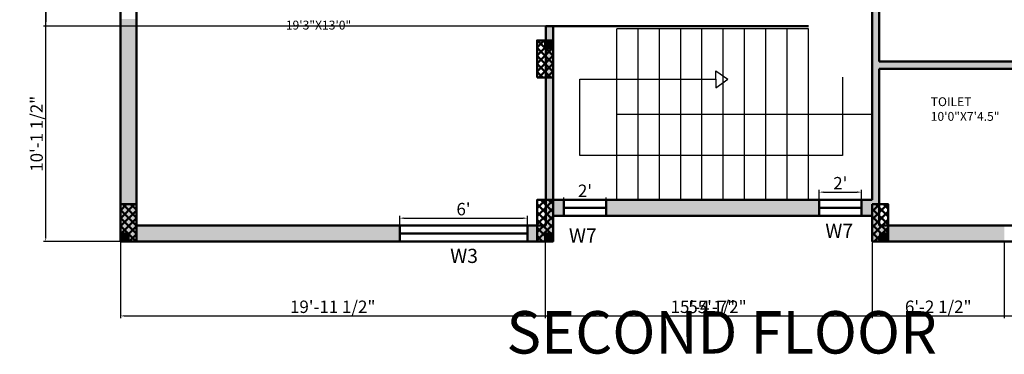
# Model space of a CAD drawing. Units: inches. Extents: x 1749 to 3550, y 1117 to 2383.
# Tile 13 of 15: x 2688 to 3244, y 1803 to 1992. Entities that reach past the tile are written whole.
import ezdxf

# ---------------------------------------------------------------- set-up
doc = ezdxf.new("R2010")
doc.units = ezdxf.units.IN
for name, color, linetype, lineweight in [('A-ANNO-DIMS', 2, 'Continuous', 18), ('A-ANNO-TEXT', 3, 'Continuous', 18), ('A-AREA-IDEN', 7, 'Continuous', 18), ('A-COLS', 10, 'Continuous', 50), ('A-FLOR-STRS', 53, 'Continuous', 25), ('A-WALL', 7, 'Continuous', 50), ('A-WALL-PATT', 8, 'Continuous', 13)]:
    doc.layers.add(name, color=color, linetype=linetype, lineweight=lineweight)
doc.styles.get("Standard").update_dxf_attribs({"font": 'arial.ttf'})
doc.dimstyles.new('ISO-25', dxfattribs={"dimtxt": 7, "dimasz": 2.5, "dimexe": 1.25, "dimexo": 0.625, "dimtad": 1, "dimdec": 1, "dimlunit": 3, "dimtxsty": 'Standard', "dimcen": 2.5, "dimadec": 0, "dimazin": 0, "dimtfac": 1, "dimtdec": 1, "dimtmove": 0, "dimatfit": 3, "dimfxl": 1, "dimarcsym": 0})

# ---------------------------------------------------------------- blocks, each defined once
blk = doc.blocks.new('*D131')
at = {"layer": 'A-ANNO-DIMS', "color": 0, "lineweight": -2, "ltscale": 0.5, "transparency": 16777216}
for p, q in [((2902.72, 1876.81), (2902.72, 1881.53)), ((2905.22, 1880.28), (2972.22, 1880.28)), ((2974.72, 1876.81), (2974.72, 1881.53))]:
    blk.add_line(p, q, dxfattribs=at)
at = {"layer": 'A-ANNO-DIMS', "color": 0, "ltscale": 0.5, "transparency": 16777216}
for points in [[(2905.22, 1880.7), (2905.22, 1879.86), (2902.72, 1880.28)], [(2972.22, 1880.7), (2972.22, 1879.86), (2974.72, 1880.28)]]:
    blk.add_solid(points, dxfattribs=at)
at = {"layer": 'Defpoints', "color": 0, "ltscale": 0.5, "transparency": 16777216}
for p in [(2974.72, 1880.28), (2902.72, 1876.18), (2974.72, 1876.18)]:
    blk.add_point(p, dxfattribs=at)
at = {"layer": 'A-ANNO-DIMS', "color": 0, "ltscale": 0.5, "transparency": 16777216, "insert": (2938.72, 1884.48), "char_height": 7, "attachment_point": 5}
blk.add_mtext("6'", dxfattribs=at)
blk = doc.blocks.new('*D132')
at = {"layer": 'A-ANNO-DIMS', "color": 0, "lineweight": -2, "ltscale": 0.5, "transparency": 16777216}
for p, q in [((2995.22, 1891.31), (2995.22, 1891.93)), ((2997.72, 1890.68), (3016.72, 1890.68)), ((3019.22, 1891.31), (3019.22, 1891.93))]:
    blk.add_line(p, q, dxfattribs=at)
at = {"layer": 'A-ANNO-DIMS', "color": 0, "ltscale": 0.5, "transparency": 16777216}
for points in [[(2997.72, 1891.1), (2997.72, 1890.26), (2995.22, 1890.68)], [(3016.72, 1891.1), (3016.72, 1890.26), (3019.22, 1890.68)]]:
    blk.add_solid(points, dxfattribs=at)
at = {"layer": 'Defpoints', "color": 0, "ltscale": 0.5, "transparency": 16777216}
for p in [(2995.22, 1890.68), (3019.22, 1890.68), (3019.22, 1890.68)]:
    blk.add_point(p, dxfattribs=at)
at = {"layer": 'A-ANNO-DIMS', "color": 0, "ltscale": 0.5, "transparency": 16777216, "insert": (3007.22, 1894.82), "char_height": 7, "attachment_point": 5}
blk.add_mtext("2'", dxfattribs=at)
blk = doc.blocks.new('*D133')
at = {"layer": 'A-ANNO-DIMS', "color": 0, "lineweight": -2, "ltscale": 0.5, "transparency": 16777216}
for p, q in [((3139.22, 1891.31), (3139.22, 1896.23)), ((3141.72, 1894.98), (3160.72, 1894.98)), ((3163.22, 1891.31), (3163.22, 1896.23))]:
    blk.add_line(p, q, dxfattribs=at)
at = {"layer": 'A-ANNO-DIMS', "color": 0, "ltscale": 0.5, "transparency": 16777216}
for points in [[(3141.72, 1895.39), (3141.72, 1894.56), (3139.22, 1894.98)], [(3160.72, 1895.39), (3160.72, 1894.56), (3163.22, 1894.98)]]:
    blk.add_solid(points, dxfattribs=at)
at = {"layer": 'Defpoints', "color": 0, "ltscale": 0.5, "transparency": 16777216}
for p in [(3163.22, 1894.98), (3139.22, 1890.68), (3163.22, 1890.68)]:
    blk.add_point(p, dxfattribs=at)
at = {"layer": 'A-ANNO-DIMS', "color": 0, "ltscale": 0.5, "transparency": 16777216, "insert": (3151.22, 1899.12), "char_height": 7, "attachment_point": 5}
blk.add_mtext("2'", dxfattribs=at)
blk = doc.blocks.new('*D180')
at = {"layer": 'A-ANNO-DIMS', "color": 0, "lineweight": -2, "ltscale": 0.5, "transparency": 16777216}
for p, q in [((2745.22, 1866.56), (2745.22, 1823.83)), ((3412.22, 1866.56), (3412.22, 1823.83)), ((2747.72, 1825.08), (3409.72, 1825.08))]:
    blk.add_line(p, q, dxfattribs=at)
at = {"layer": 'A-ANNO-DIMS', "color": 0, "ltscale": 0.5, "transparency": 16777216}
for points in [[(2747.72, 1825.5), (2747.72, 1824.66), (2745.22, 1825.08)], [(3409.72, 1825.5), (3409.72, 1824.66), (3412.22, 1825.08)]]:
    blk.add_solid(points, dxfattribs=at)
at = {"layer": 'Defpoints', "color": 0, "ltscale": 0.5, "transparency": 16777216}
for p in [(2745.22, 1867.18), (3412.22, 1867.18), (3412.22, 1825.08)]:
    blk.add_point(p, dxfattribs=at)
at = {"layer": 'A-ANNO-DIMS', "color": 0, "ltscale": 0.5, "transparency": 16777216, "insert": (3078.72, 1829.27), "char_height": 7, "attachment_point": 5}
blk.add_mtext('55\'-7"', dxfattribs=at)
blk = doc.blocks.new('*D181')
at = {"layer": 'A-ANNO-DIMS', "color": 0, "lineweight": -2, "ltscale": 0.5, "transparency": 16777216}
for p, q in [((2744.59, 2309.68), (2701.86, 2309.68)), ((2703.11, 1869.68), (2703.11, 2307.18)), ((2744.59, 1867.18), (2701.86, 1867.18))]:
    blk.add_line(p, q, dxfattribs=at)
at = {"layer": 'A-ANNO-DIMS', "color": 0, "ltscale": 0.5, "transparency": 16777216}
for points in [[(2702.69, 2307.18), (2703.52, 2307.18), (2703.11, 2309.68)], [(2702.69, 1869.68), (2703.52, 1869.68), (2703.11, 1867.18)]]:
    blk.add_solid(points, dxfattribs=at)
at = {"layer": 'Defpoints', "color": 0, "ltscale": 0.5, "transparency": 16777216}
for p in [(2703.11, 2309.68), (2745.22, 2309.68), (2745.22, 1867.18)]:
    blk.add_point(p, dxfattribs=at)
at = {"layer": 'A-ANNO-DIMS', "color": 0, "ltscale": 0.5, "transparency": 16777216, "insert": (2698.86, 2088.43), "char_height": 7, "attachment_point": 5, "rotation": 90}
blk.add_mtext('36\'-10 1/2"', dxfattribs=at)
blk = doc.blocks.new('*D184')
at = {"layer": 'A-ANNO-DIMS', "color": 0, "lineweight": -2, "ltscale": 0.5, "transparency": 16777216}
for p, q in [((2745.22, 1866.56), (2745.22, 1823.83)), ((2984.72, 1866.56), (2984.72, 1823.83)), ((2747.72, 1825.08), (2982.22, 1825.08))]:
    blk.add_line(p, q, dxfattribs=at)
at = {"layer": 'A-ANNO-DIMS', "color": 0, "ltscale": 0.5, "transparency": 16777216}
for points in [[(2747.72, 1825.5), (2747.72, 1824.66), (2745.22, 1825.08)], [(2982.22, 1825.5), (2982.22, 1824.66), (2984.72, 1825.08)]]:
    blk.add_solid(points, dxfattribs=at)
at = {"layer": 'Defpoints', "color": 0, "ltscale": 0.5, "transparency": 16777216}
for p in [(2745.22, 1867.18), (2984.72, 1867.18), (2984.72, 1825.08)]:
    blk.add_point(p, dxfattribs=at)
at = {"layer": 'A-ANNO-DIMS', "color": 0, "ltscale": 0.5, "transparency": 16777216, "insert": (2864.97, 1829.33), "char_height": 7, "attachment_point": 5}
blk.add_mtext('19\'-11 1/2"', dxfattribs=at)
blk = doc.blocks.new('*D185')
at = {"layer": 'A-ANNO-DIMS', "color": 0, "lineweight": -2, "ltscale": 0.5, "transparency": 16777216}
for p, q in [((2984.72, 1866.56), (2984.72, 1823.83)), ((3169.22, 1866.56), (3169.22, 1823.83)), ((2987.22, 1825.08), (3166.72, 1825.08))]:
    blk.add_line(p, q, dxfattribs=at)
at = {"layer": 'A-ANNO-DIMS', "color": 0, "ltscale": 0.5, "transparency": 16777216}
for points in [[(2987.22, 1825.5), (2987.22, 1824.66), (2984.72, 1825.08)], [(3166.72, 1825.5), (3166.72, 1824.66), (3169.22, 1825.08)]]:
    blk.add_solid(points, dxfattribs=at)
at = {"layer": 'Defpoints', "color": 0, "ltscale": 0.5, "transparency": 16777216}
for p in [(2984.72, 1867.18), (3169.22, 1867.18), (3169.22, 1825.08)]:
    blk.add_point(p, dxfattribs=at)
at = {"layer": 'A-ANNO-DIMS', "color": 0, "ltscale": 0.5, "transparency": 16777216, "insert": (3076.97, 1829.33), "char_height": 7, "attachment_point": 5}
blk.add_mtext('15\'-4 1/2"', dxfattribs=at)
blk = doc.blocks.new('*D186')
at = {"layer": 'A-ANNO-DIMS', "color": 0, "lineweight": -2, "ltscale": 0.5, "transparency": 16777216}
for p, q in [((3169.22, 1866.56), (3169.22, 1823.83)), ((3243.72, 1866.56), (3243.72, 1823.83)), ((3171.72, 1825.08), (3241.22, 1825.08))]:
    blk.add_line(p, q, dxfattribs=at)
at = {"layer": 'A-ANNO-DIMS', "color": 0, "ltscale": 0.5, "transparency": 16777216}
for points in [[(3171.72, 1825.5), (3171.72, 1824.66), (3169.22, 1825.08)], [(3241.22, 1825.5), (3241.22, 1824.66), (3243.72, 1825.08)]]:
    blk.add_solid(points, dxfattribs=at)
at = {"layer": 'Defpoints', "color": 0, "ltscale": 0.5, "transparency": 16777216}
for p in [(3169.22, 1867.18), (3243.72, 1867.18), (3243.72, 1825.08)]:
    blk.add_point(p, dxfattribs=at)
at = {"layer": 'A-ANNO-DIMS', "color": 0, "ltscale": 0.5, "transparency": 16777216, "insert": (3206.47, 1829.33), "char_height": 7, "attachment_point": 5}
blk.add_mtext('6\'-2 1/2"', dxfattribs=at)
blk = doc.blocks.new('*D194')
at = {"layer": 'A-ANNO-DIMS', "color": 0, "lineweight": -2, "ltscale": 0.5, "transparency": 16777216}
for p, q in [((2988.59, 2028.68), (2701.86, 2028.68)), ((2703.11, 2026.18), (2703.11, 1991.18)), ((2988.59, 1988.68), (2701.86, 1988.68))]:
    blk.add_line(p, q, dxfattribs=at)
at = {"layer": 'A-ANNO-DIMS', "color": 0, "ltscale": 0.5, "transparency": 16777216}
for points in [[(2702.69, 2026.18), (2703.52, 2026.18), (2703.11, 2028.68)], [(2702.69, 1991.18), (2703.52, 1991.18), (2703.11, 1988.68)]]:
    blk.add_solid(points, dxfattribs=at)
at = {"layer": 'Defpoints', "color": 0, "ltscale": 0.5, "transparency": 16777216}
for p in [(2989.22, 2028.68), (2703.11, 1988.68), (2989.22, 1988.68)]:
    blk.add_point(p, dxfattribs=at)
at = {"layer": 'A-ANNO-DIMS', "color": 0, "ltscale": 0.5, "transparency": 16777216, "insert": (2698.91, 2008.68), "char_height": 7, "attachment_point": 5, "rotation": 90}
blk.add_mtext('3\'-4"', dxfattribs=at)
blk = doc.blocks.new('*D198')
at = {"layer": 'A-ANNO-DIMS', "color": 0, "lineweight": -2, "ltscale": 0.5, "transparency": 16777216}
for p, q in [((2988.59, 1988.68), (2701.86, 1988.68)), ((2703.11, 1869.68), (2703.11, 1986.18)), ((2988.59, 1867.18), (2701.86, 1867.18))]:
    blk.add_line(p, q, dxfattribs=at)
at = {"layer": 'A-ANNO-DIMS', "color": 0, "ltscale": 0.5, "transparency": 16777216}
for points in [[(2702.69, 1986.18), (2703.52, 1986.18), (2703.11, 1988.68)], [(2702.69, 1869.68), (2703.52, 1869.68), (2703.11, 1867.18)]]:
    blk.add_solid(points, dxfattribs=at)
at = {"layer": 'Defpoints', "color": 0, "ltscale": 0.5, "transparency": 16777216}
for p in [(2703.11, 1988.68), (2989.22, 1988.68), (2989.22, 1867.18)]:
    blk.add_point(p, dxfattribs=at)
at = {"layer": 'A-ANNO-DIMS', "color": 0, "ltscale": 0.5, "transparency": 16777216, "insert": (2698.86, 1927.93), "char_height": 7, "attachment_point": 5, "rotation": 90}
blk.add_mtext('10\'-1 1/2"', dxfattribs=at)

msp = doc.modelspace()

# ---------------------------------------------------------------- hatches: boundary and pattern name
at = {"layer": 'A-COLS', "ltscale": 10}
h = msp.add_hatch(dxfattribs=at)
h.set_pattern_fill('ANSI37', color=256, angle=90)
h.set_pattern_definition([(135, (4347.3257, 308.4367), (-2.245064, -2.245064), []), (225, (4347.3257, 308.4367), (2.245064, -2.245064), [])])
h.paths.add_polyline_path([(2989.22, 1980.68), (2980.22, 1980.68), (2980.22, 1959.68), (2989.22, 1959.68)])
h = msp.add_hatch(color=256, dxfattribs=at)
h.dxf.hatch_style = 1
h.paths.add_polyline_path([(2984.72, 1980.68), (2984.72, 1976.18), (2989.22, 1976.18), (2989.22, 1980.68)])
h = msp.add_hatch(dxfattribs=at)
h.set_pattern_fill('ANSI37', color=256, angle=270)
h.set_pattern_definition([(315, (1387.1136, 3539.4255), (2.245064, 2.245064), []), (45, (1387.1136, 3539.4255), (-2.245064, 2.245064), [])])
h.paths.add_polyline_path([(2745.22, 1867.18), (2754.22, 1867.18), (2754.22, 1888.18), (2745.22, 1888.18)])
h = msp.add_hatch(dxfattribs=at)
h.set_pattern_fill('ANSI37', color=256, angle=270)
h.set_pattern_definition([(315, (1602.912, 3539.4255), (2.245064, 2.245064), []), (45, (1602.912, 3539.4255), (-2.245064, 2.245064), [])])
h.paths.add_polyline_path([(2989.22, 1890.68), (2980.22, 1890.68), (2980.22, 1867.18), (2989.22, 1867.18)])
h = msp.add_hatch(dxfattribs=at)
h.set_pattern_fill('ANSI37', color=256, angle=270)
h.set_pattern_definition([(315, (1829.7387, 3539.4255), (2.245064, 2.245064), []), (45, (1829.7387, 3539.4255), (-2.245064, 2.245064), [])])
h.paths.add_polyline_path([(3178.22, 1888.18), (3169.22, 1888.18), (3169.22, 1867.18), (3178.22, 1867.18)])
h = msp.add_hatch(color=256, dxfattribs=at)
h.dxf.hatch_style = 1
h.paths.add_polyline_path([(2749.72, 1867.18), (2749.72, 1871.68), (2745.22, 1871.68), (2745.22, 1867.18)])
h = msp.add_hatch(color=256, dxfattribs=at)
h.dxf.hatch_style = 1
h.paths.add_polyline_path([(2989.22, 1867.18), (2989.22, 1871.68), (2984.72, 1871.68), (2984.72, 1867.18)])
h = msp.add_hatch(color=256, dxfattribs=at)
h.dxf.hatch_style = 1
h.paths.add_polyline_path([(3178.22, 1867.18), (3178.22, 1871.68), (3173.72, 1871.68), (3173.72, 1867.18)])
at = {"layer": 'A-WALL-PATT', "ltscale": 0.5}
h = msp.add_hatch(color=256, dxfattribs=at)
h.dxf.hatch_style = 1
h.paths.add_polyline_path([(3303.22, 1968.68), (3289.22, 1968.68), (3173.22, 1968.68), (3173.22, 2053.68), (3169.22, 2053.68), (3169.22, 1964.68), (3169.22, 1890.68), (3163.22, 1890.68), (3163.22, 1881.68), (3169.22, 1881.68), (3169.22, 1867.18), (3243.72, 1867.18), (3243.72, 1876.18), (3173.22, 1876.18), (3173.22, 1964.68), (3289.22, 1964.68), (3293.22, 1964.68), (3293.22, 1958.68), (3297.22, 1958.68), (3297.22, 1964.68), (3303.22, 1964.68)])
h = msp.add_hatch(color=256, dxfattribs=at)
h.dxf.hatch_style = 1
h.paths.add_polyline_path([(2754.22, 1876.18), (2754.22, 1992.68), (2745.22, 1992.68), (2745.22, 1881.68), (2745.22, 1867.18), (2902.72, 1867.18), (2902.72, 1876.18)])
h = msp.add_hatch(color=256, dxfattribs=at)
h.dxf.hatch_style = 1
h.paths.add_polyline_path([(2985.22, 1890.68), (2985.22, 1876.18), (2974.72, 1876.18), (2974.72, 1867.18), (2989.22, 1867.18), (2989.22, 1881.68), (2995.22, 1881.68), (2995.22, 1890.68), (2989.22, 1890.68), (2989.22, 1988.68), (2985.22, 1988.68)])
h = msp.add_hatch(color=256, dxfattribs=at)
h.dxf.hatch_style = 1
h.paths.add_polyline_path([(3139.22, 1881.68), (3139.22, 1890.68), (3019.22, 1890.68), (3019.22, 1881.68)])

# ---------------------------------------------------------------- linework, layer by layer
at = {"layer": 'A-COLS', "ltscale": 10}
for points in [[(2980.22, 1959.68), (2980.22, 1980.68), (2989.22, 1980.68), (2989.22, 1959.68)], [(2984.72, 1980.68), (2989.22, 1980.68), (2989.22, 1976.18), (2984.72, 1976.18)], [(2754.22, 1888.18), (2754.22, 1867.18), (2745.22, 1867.18), (2745.22, 1888.18)], [(2980.22, 1890.68), (2980.22, 1867.18), (2989.22, 1867.18), (2989.22, 1890.68)], [(3169.22, 1888.18), (3169.22, 1867.18), (3178.22, 1867.18), (3178.22, 1888.18)], [(2749.72, 1867.18), (2745.22, 1867.18), (2745.22, 1871.68), (2749.72, 1871.68)], [(2984.72, 1867.18), (2989.22, 1867.18), (2989.22, 1871.68), (2984.72, 1871.68)], [(3173.72, 1867.18), (3178.22, 1867.18), (3178.22, 1871.68), (3173.72, 1871.68)]]:
    msp.add_lwpolyline(points, close=True, dxfattribs=at)
at = {"layer": 'A-FLOR-STRS', "ltscale": 0.5}
for p, q in [((3133.22, 1987.18), (3025.22, 1987.18)), ((3025.22, 1890.68), (3025.22, 1987.18)), ((3037.22, 1890.68), (3037.22, 1987.18)), ((3049.22, 1890.68), (3049.22, 1987.18)), ((3061.22, 1890.68), (3061.22, 1987.18)), ((3073.22, 1890.68), (3073.22, 1987.18)), ((3085.22, 1890.68), (3085.22, 1987.18)), ((3097.22, 1890.68), (3097.22, 1987.18)), ((3109.22, 1890.68), (3109.22, 1987.18)), ((3121.22, 1890.68), (3121.22, 1987.18)), ((3133.22, 1890.68), (3133.22, 1987.18)), ((3133.22, 1890.68), (3133.22, 1987.18)), ((3081.08, 1958.72), (3081.08, 1963.48)), ((3081.08, 1963.48), (3087.76, 1958.72)), ((3004.3, 1915.59), (3004.3, 1958.72)), ((3004.3, 1958.72), (3081.08, 1958.72)), ((3081.08, 1958.72), (3081.08, 1953.95)), ((3081.08, 1953.95), (3087.76, 1958.72)), ((3152.43, 1959.83), (3152.43, 1915.59)), ((3025.22, 1938.93), (3169.22, 1938.93)), ((3152.43, 1915.59), (3004.3, 1915.59)), ((2989.22, 1890.68), (3025.22, 1890.68)), ((3169.22, 1890.68), (3133.22, 1890.68))]:
    msp.add_line(p, q, dxfattribs=at)
at = {"layer": 'A-WALL', "ltscale": 0.5}
for p, q in [((2745.22, 2309.68), (2745.22, 1881.68)), ((3169.22, 2053.68), (3169.22, 1964.68)), ((3173.22, 2053.68), (3173.22, 1968.68)), ((2754.22, 2046.68), (2754.22, 1876.18)), ((2985.22, 1988.68), (2989.22, 1988.68)), ((2985.22, 1988.68), (2985.22, 1890.68)), ((2989.22, 1988.68), (2989.22, 1890.68)), ((2989.22, 1988.68), (3133.22, 1988.68)), ((2985.22, 1980.68), (2989.22, 1980.68)), ((3173.22, 1968.68), (3289.22, 1968.68)), ((3169.22, 1964.68), (3169.22, 1890.68)), ((3173.22, 1964.68), (3289.22, 1964.68)), ((3173.22, 1964.68), (3173.22, 1876.18)), ((2985.22, 1890.68), (2985.22, 1876.18)), ((2989.22, 1890.68), (3169.22, 1890.68)), ((2995.22, 1881.68), (2995.22, 1890.68)), ((3019.22, 1881.68), (3019.22, 1890.68)), ((3139.22, 1881.68), (3139.22, 1890.68)), ((3163.22, 1881.68), (3163.22, 1890.68)), ((2995.22, 1886.18), (3019.22, 1886.18)), ((3139.22, 1886.18), (3163.22, 1886.18)), ((2745.22, 1881.68), (2745.22, 1867.18)), ((2989.22, 1881.68), (3169.22, 1881.68)), ((2989.22, 1881.68), (2989.22, 1867.18)), ((3169.22, 1881.68), (3169.22, 1867.18)), ((2985.22, 1876.18), (2754.22, 1876.18)), ((2902.72, 1876.18), (2902.72, 1867.18)), ((2902.72, 1871.68), (2974.72, 1871.68)), ((2974.72, 1876.18), (2974.72, 1867.18)), ((3173.22, 1876.18), (3293.22, 1876.18)), ((2955.83, 1867.18), (2745.22, 1867.18)), ((2989.22, 1867.18), (2955.83, 1867.18)), ((3169.22, 1867.18), (3412.22, 1867.18))]:
    msp.add_line(p, q, dxfattribs=at)

# ---------------------------------------------------------------- texts
at = {"layer": 'A-ANNO-TEXT', "ltscale": 0.5}
for s, height, p in [('W7', 8, (3142.79, 1869.14)), ('W7', 8, (2998.19, 1866.47)), ('W3', 8, (2931.22, 1854.98)), ('SECOND FLOOR', 24, (2962.96, 1803.81))]:
    msp.add_text(s, height=height, dxfattribs=at).set_placement(p)
at = {"layer": 'A-AREA-IDEN', "ltscale": 0.5}
for s, p in [('19\'3"X13\'0"', (2838.52, 1986.8)), ('TOILET', (3202.23, 1943.55)), ('10\'0"X7\'4.5"', (3202.23, 1935.25))]:
    msp.add_text(s, height=5, dxfattribs=at).set_placement(p)

# ---------------------------------------------------------------- dimensions: what is measured, and where the dimension line sits
at = {"layer": 'A-ANNO-DIMS', "ltscale": 0.5}
for base, p1, p2, picture, middle in [((2703.11, 2309.68), (2745.22, 1867.18), (2745.22, 2309.68), '*D181', (2698.86, 2088.43)), ((2703.11, 1988.68), (2989.22, 2028.68), (2989.22, 1988.68), '*D194', (2698.91, 2008.68)), ((2703.11, 1988.68), (2989.22, 1867.18), (2989.22, 1988.68), '*D198', (2698.86, 1927.93))]:
    dim = msp.add_linear_dim(base=base, p1=p1, p2=p2, angle=90, dimstyle='ISO-25', override={"dimdec": 1, "dimlfac": 1, "dimrnd": 0, "dimzin": 1, "dimdsep": 46, "dimlunit": 4, "dimfrac": 2}, dxfattribs=at)
    dim.commit()
    dim.dimension.update_dxf_attribs({"geometry": picture, "text_midpoint": middle})
for base, p1, p2, override, picture, middle in [((3019.22, 1890.68), (2995.22, 1890.68), (3019.22, 1890.68), {"dimclrd": 0, "dimclre": 0, "dimclrt": 0}, '*D132', (3007.22, 1894.82)), ((3163.22, 1894.98), (3139.22, 1890.68), (3163.22, 1890.68), {"dimclrd": 0, "dimclre": 0, "dimclrt": 0}, '*D133', (3151.22, 1899.12)), ((2974.72, 1880.28), (2902.72, 1876.18), (2974.72, 1876.18), {"dimclrd": 0, "dimclre": 0, "dimclrt": 0}, '*D131', (2938.72, 1884.48)), ((3412.22, 1825.08), (2745.22, 1867.18), (3412.22, 1867.18), {"dimdec": 1, "dimlfac": 1, "dimrnd": 0, "dimzin": 1, "dimdsep": 46, "dimlunit": 4, "dimfrac": 2}, '*D180', (3078.72, 1829.27)), ((2984.72, 1825.08), (2745.22, 1867.18), (2984.72, 1867.18), {"dimdec": 1, "dimlfac": 1, "dimrnd": 0, "dimzin": 1, "dimdsep": 46, "dimlunit": 4, "dimfrac": 2}, '*D184', (2864.97, 1829.33)), ((3169.22, 1825.08), (2984.72, 1867.18), (3169.22, 1867.18), {"dimdec": 1, "dimlfac": 1, "dimrnd": 0, "dimzin": 1, "dimdsep": 46, "dimlunit": 4, "dimfrac": 2}, '*D185', (3076.97, 1829.33)), ((3243.72, 1825.08), (3169.22, 1867.18), (3243.72, 1867.18), {"dimdec": 1, "dimlfac": 1, "dimrnd": 0, "dimzin": 1, "dimdsep": 46, "dimlunit": 4, "dimfrac": 2}, '*D186', (3206.47, 1829.33))]:
    dim = msp.add_linear_dim(base=base, p1=p1, p2=p2, dimstyle='ISO-25', override=override, dxfattribs=at)
    dim.commit()
    dim.dimension.update_dxf_attribs({"geometry": picture, "text_midpoint": middle})

doc.saveas('drawing.dxf')
